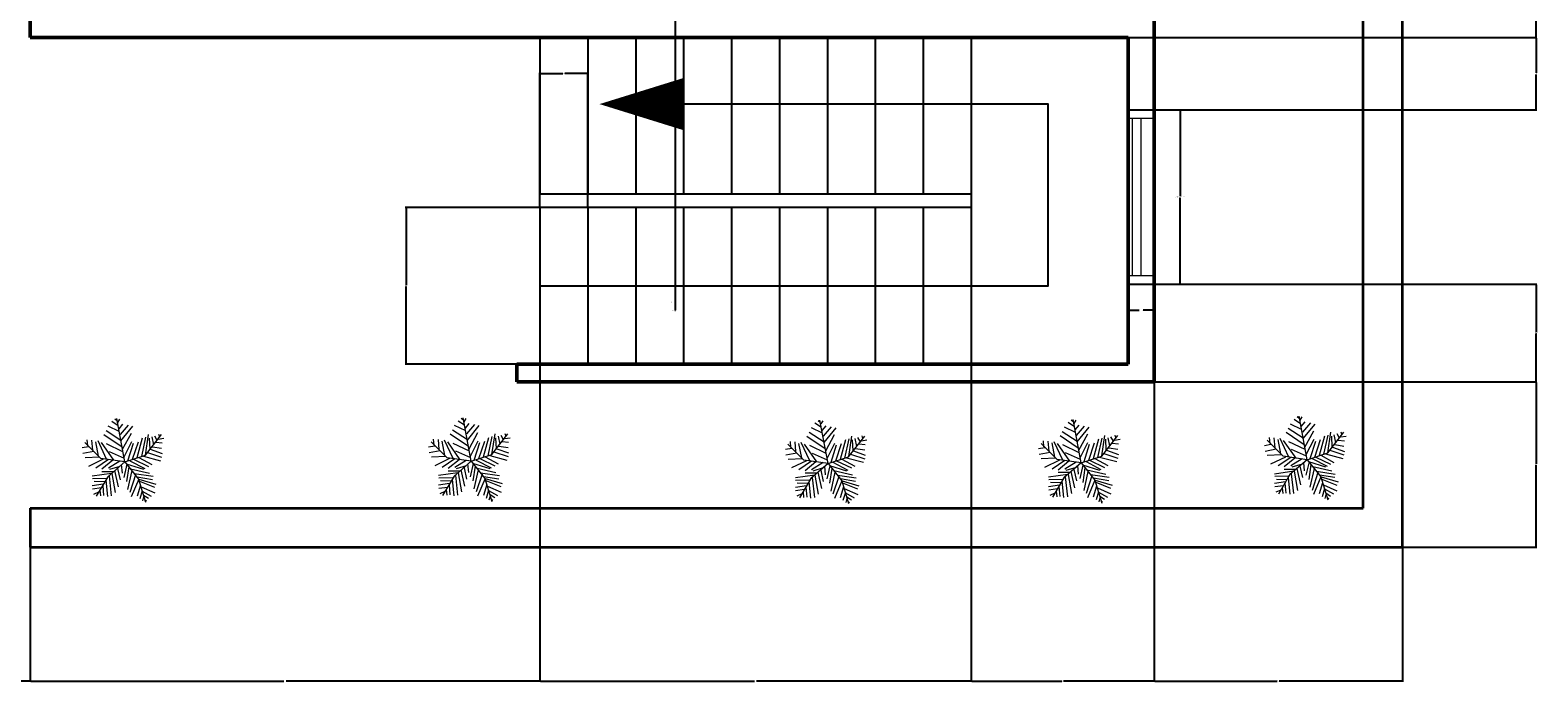
# Model space of a CAD drawing. Units: inches. Extents: x 156 to 720, y 11 to 679.
# Tile 2 of 5: x 374 to 720, y 11 to 161. Entities that reach past the tile are written whole.
import ezdxf

# ---------------------------------------------------------------- set-up
doc = ezdxf.new("R2010")
doc.units = ezdxf.units.IN
for name, color, linetype, lineweight in [('A-ANNO-DIMS', 2, 'Continuous', 18), ('A-FLOR-STRS', 7, 'Continuous', 25), ('A-GLAZ', 4, 'Continuous', 18), ('A-WALL', 7, 'Continuous', 50), ('C-PROP', 7, 'Continuous', 35), ('L-PLNT', 94, 'Continuous', 13)]:
    doc.layers.add(name, color=color, linetype=linetype, lineweight=lineweight)
doc.styles.get("Standard").update_dxf_attribs({"font": 'arial.ttf'})
doc.dimstyles.get("Standard").update_dxf_attribs({"dimtxt": 0.18, "dimasz": 0.18, "dimexe": 0.18, "dimexo": 0.0625, "dimgap": 0.09, "dimtad": 0, "dimtih": 1, "dimtoh": 1, "dimdec": 4, "dimzin": 0, "dimdsep": 46, "dimtxsty": 'Standard', "dimcen": 0.09, "dimadec": 0, "dimazin": 0, "dimtfac": 1, "dimtdec": 4, "dimtofl": 0, "dimtmove": 0, "dimatfit": 3, "dimfxl": 1, "dimtolj": 1, "dimtzin": 0, "dimarcsym": 0})

# ---------------------------------------------------------------- blocks, each defined once
blk = doc.blocks.new('*U13')
for p, q in [((-5.114, 28.097), (-24.676, 40.636)), ((-7.288, 39.707), (-21.778, 46.673)), ((-8.737, 47.138), (-17.069, 52.711)), ((-10.186, 53.64), (-13.084, 55.962)), ((0, 0), (-10.5, 57)), ((-9.099, 51.782), (-6.563, 55.962)), ((-7.65, 43.423), (-2.578, 49.46)), ((-5.839, 35.992), (4.667, 48.067)), ((-5.114, 27.632), (10.463, 46.673)), ((-31.5, 4.5), (-52.5, 25.5)), ((-48.585, 21.131), (-49.309, 29.026)), ((-43.513, 28.561), (-42.427, 15.558)), ((-38.442, 26.239), (-34.819, 7.663)), ((-35.544, 28.097), (-24.314, 3.947)), ((-14.533, 2.09), (-30.834, 25.31)), ((-3.665, 19.273), (-27.574, 35.527)), ((-24.314, 23.917), (-2.941, 13.7)), ((-2.941, 16.486), (8.652, 37.85)), ((-1.129, 6.734), (9.014, 26.704)), ((3.942, 1.625), (11.187, 24.381)), ((10.101, 3.483), (17.708, 26.239)), ((16.259, 5.805), (23.142, 31.348)), ((22.055, 7.198), (27.489, 32.277)), ((27, 9), (48, 36)), ((27.127, 9.056), (31.112, 35.992)), ((31.836, 30.883), (32.561, 16.486)), ((35.096, 32.741), (37.27, 22.524)), ((38.719, 34.134), (41.979, 28.561)), ((40.53, 25.775), (48.862, 24.846)), ((43.791, 29.954), (51.036, 30.883)), ((44.153, 36.456), (45.239, 32.741)), ((-47.498, 19.737), (-55.83, 18.344)), ((-40.615, 13.7), (-55.105, 10.913)), ((-33.37, 6.269), (-52.207, 5.34)), ((-28.299, 3.483), (-47.86, -5.805)), ((-21.416, 3.018), (-38.079, -8.128)), ((0, 0), (-31.5, 4.5)), ((-15.982, 2.09), (-30.11, -9.521)), ((0, 0), (-22.5, -19.5)), ((-6.563, 1.161), (-21.416, -8.128)), ((-20.691, 13.7), (-1.129, 4.876)), ((0, 0), (27, 9)), ((0, 0), (18, -22.5)), ((6.478, 1.625), (26.04, -8.592)), ((11.187, 3.483), (30.749, -5.805)), ((18.07, 5.805), (35.096, -3.483)), ((24.229, 7.663), (46.688, 1.625)), ((29.662, 12.307), (48.137, 6.269)), ((33.285, 16.486), (48.862, 10.913)), ((36.183, 19.737), (48.137, 17.88)), ((-17.431, -15.094), (-42.789, -18.809)), ((-22.5, -19.5), (-37.5, -45)), ((-15.257, -12.772), (-30.11, -12.772)), ((-20.691, -18.345), (-17.793, -44.352)), ((-6.563, -5.805), (-19.967, -9.985)), ((-17.069, -15.094), (-12.721, -40.172)), ((-13.446, -11.378), (-8.737, -32.741)), ((-9.461, -8.592), (-6.201, -23.453)), ((-4.752, -3.483), (-3.665, -14.629)), ((2.493, -3.019), (-1.491, -20.202)), ((1.769, -2.555), (24.229, -9.521)), ((5.029, -6.27), (2.131, -25.775)), ((9.014, -11.378), (3.58, -35.992)), ((14.085, -16.951), (6.478, -40.172)), ((7.565, -9.056), (32.198, -14.629)), ((12.274, -15.094), (36.907, -18.809)), ((16.259, -19.738), (36.183, -22.989)), ((-28.299, -29.026), (-42.789, -31.348)), ((-24.314, -21.596), (-42.427, -22.06)), ((-30.834, -34.135), (-42.427, -35.528)), ((-26.849, -26.24), (-40.253, -25.775)), ((-32.646, -36.921), (-31.921, -44.352)), ((-29.023, -30.884), (-27.936, -43.887)), ((-25.038, -23.918), (-22.865, -45.281)), ((18.07, -22.524), (8.289, -45.745)), ((20.244, -30.419), (15.897, -44.816)), ((18, -22.5), (27, -52.5)), ((18.433, -22.524), (40.53, -29.026)), ((19.157, -25.311), (38.719, -33.206)), ((22.78, -37.85), (19.519, -48.532)), ((21.331, -32.741), (39.081, -40.636)), ((22.78, -38.314), (34.372, -44.816)), ((-34.457, -39.708), (-40.978, -42.494)), ((24.591, -45.745), (23.142, -50.854)), ((24.591, -43.423), (30.749, -47.603)), ((26.764, -49.925), (28.213, -50.854))]:
    blk.add_line(p, q)
blk = doc.blocks.new('WIN-36IN-WALL6')
for p, q in [((6, 40), (0, 40)), ((6, 38), (0, 38)), ((0, 38), (0, 2)), ((1, 2), (1, 38)), ((3, 2), (3, 38)), ((6, 2), (6, 38)), ((0, 2), (6, 2)), ((0, 0), (6, 0))]:
    blk.add_line(p, q)
blk = doc.blocks.new('*D33')
at = {"layer": 'A-ANNO-DIMS', "color": 0, "lineweight": -2, "transparency": 16777216}
for p, q in [((631.79, 142.54), (637.9, 142.54)), ((637.72, 142.36), (637.72, 122.73)), ((637.72, 102.72), (637.72, 122.36)), ((631.79, 102.54), (637.9, 102.54))]:
    blk.add_line(p, q, dxfattribs=at)
at = {"layer": 'A-ANNO-DIMS', "color": 0, "transparency": 16777216}
for points in [[(637.69, 142.36), (637.75, 142.36), (637.72, 142.54)], [(637.69, 102.72), (637.75, 102.72), (637.72, 102.54)]]:
    blk.add_solid(points, dxfattribs=at)
at = {"layer": 'Defpoints', "color": 0, "transparency": 16777216}
for p in [(631.72, 142.54), (637.72, 142.54), (631.72, 102.54)]:
    blk.add_point(p, dxfattribs=at)
at = {"layer": 'A-ANNO-DIMS', "color": 0, "transparency": 16777216, "insert": (637.72, 122.54), "char_height": 0.18, "attachment_point": 5}
blk.add_mtext('\\A1;WINDOW C 40 TYP.', dxfattribs=at)
blk = doc.blocks.new('*D34')
at = {"layer": 'A-ANNO-DIMS', "color": 0, "lineweight": -2, "transparency": 16777216}
for p, q in [((625.72, 102.48), (625.72, 96.36)), ((631.72, 102.48), (631.72, 96.36)), ((625.9, 96.54), (628.26, 96.54)), ((631.54, 96.54), (629.18, 96.54))]:
    blk.add_line(p, q, dxfattribs=at)
at = {"layer": 'A-ANNO-DIMS', "color": 0, "transparency": 16777216}
for points in [[(625.9, 96.57), (625.9, 96.51), (625.72, 96.54)], [(631.54, 96.57), (631.54, 96.51), (631.72, 96.54)]]:
    blk.add_solid(points, dxfattribs=at)
at = {"layer": 'Defpoints', "color": 0, "transparency": 16777216}
for p in [(625.72, 102.54), (631.72, 102.54), (631.72, 96.54)]:
    blk.add_point(p, dxfattribs=at)
at = {"layer": 'A-ANNO-DIMS', "color": 0, "transparency": 16777216, "insert": (628.72, 96.54), "char_height": 0.18, "attachment_point": 5}
blk.add_mtext('\\A1;6 TYP.', dxfattribs=at)
blk = doc.blocks.new('*D52')
at = {"layer": 'A-ANNO-DIMS', "color": 0, "lineweight": -2, "transparency": 16777216}
for p, q in [((241.72, 42.09), (241.72, 11.27)), ((373.72, 42.09), (373.72, 11.27)), ((241.9, 11.45), (307.44, 11.45)), ((373.54, 11.45), (308, 11.45))]:
    blk.add_line(p, q, dxfattribs=at)
at = {"layer": 'A-ANNO-DIMS', "color": 0, "transparency": 16777216}
for points in [[(241.9, 11.48), (241.9, 11.42), (241.72, 11.45)], [(373.54, 11.48), (373.54, 11.42), (373.72, 11.45)]]:
    blk.add_solid(points, dxfattribs=at)
at = {"layer": 'Defpoints', "color": 0, "transparency": 16777216}
for p in [(241.72, 42.15), (373.72, 42.15), (373.72, 11.45)]:
    blk.add_point(p, dxfattribs=at)
at = {"layer": 'A-ANNO-DIMS', "color": 0, "transparency": 16777216, "insert": (307.72, 11.45), "char_height": 0.18, "attachment_point": 5}
blk.add_mtext('\\A1;132', dxfattribs=at)
blk = doc.blocks.new('*D53')
at = {"layer": 'A-ANNO-DIMS', "color": 0, "lineweight": -2, "transparency": 16777216}
for p, q in [((490.72, 84.09), (490.72, 11.27)), ((373.72, 42.09), (373.72, 11.27)), ((373.9, 11.45), (431.94, 11.45)), ((490.54, 11.45), (432.5, 11.45))]:
    blk.add_line(p, q, dxfattribs=at)
at = {"layer": 'A-ANNO-DIMS', "color": 0, "transparency": 16777216}
for points in [[(373.9, 11.48), (373.9, 11.42), (373.72, 11.45)], [(490.54, 11.48), (490.54, 11.42), (490.72, 11.45)]]:
    blk.add_solid(points, dxfattribs=at)
at = {"layer": 'Defpoints', "color": 0, "transparency": 16777216}
for p in [(490.72, 84.15), (373.72, 42.15), (490.72, 11.45)]:
    blk.add_point(p, dxfattribs=at)
at = {"layer": 'A-ANNO-DIMS', "color": 0, "transparency": 16777216, "insert": (432.22, 11.45), "char_height": 0.18, "attachment_point": 5}
blk.add_mtext('\\A1;117', dxfattribs=at)
blk = doc.blocks.new('*D54')
at = {"layer": 'A-ANNO-DIMS', "color": 0, "lineweight": -2, "transparency": 16777216}
for p, q in [((490.72, 84.09), (490.72, 11.27)), ((589.72, 84.09), (589.72, 11.27)), ((490.9, 11.45), (540, 11.45)), ((589.54, 11.45), (540.44, 11.45))]:
    blk.add_line(p, q, dxfattribs=at)
at = {"layer": 'A-ANNO-DIMS', "color": 0, "transparency": 16777216}
for points in [[(490.9, 11.48), (490.9, 11.42), (490.72, 11.45)], [(589.54, 11.48), (589.54, 11.42), (589.72, 11.45)]]:
    blk.add_solid(points, dxfattribs=at)
at = {"layer": 'Defpoints', "color": 0, "transparency": 16777216}
for p in [(490.72, 84.15), (589.72, 84.15), (589.72, 11.45)]:
    blk.add_point(p, dxfattribs=at)
at = {"layer": 'A-ANNO-DIMS', "color": 0, "transparency": 16777216, "insert": (540.22, 11.45), "char_height": 0.18, "attachment_point": 5}
blk.add_mtext('\\A1;99', dxfattribs=at)
blk = doc.blocks.new('*D55')
at = {"layer": 'A-ANNO-DIMS', "color": 0, "lineweight": -2, "transparency": 16777216}
for p, q in [((589.72, 84.09), (589.72, 11.27)), ((631.72, 80.09), (631.72, 11.27)), ((589.9, 11.45), (610.5, 11.45)), ((631.54, 11.45), (610.95, 11.45))]:
    blk.add_line(p, q, dxfattribs=at)
at = {"layer": 'A-ANNO-DIMS', "color": 0, "transparency": 16777216}
for points in [[(589.9, 11.48), (589.9, 11.42), (589.72, 11.45)], [(631.54, 11.48), (631.54, 11.42), (631.72, 11.45)]]:
    blk.add_solid(points, dxfattribs=at)
at = {"layer": 'Defpoints', "color": 0, "transparency": 16777216}
for p in [(589.72, 84.15), (631.72, 80.15), (631.72, 11.45)]:
    blk.add_point(p, dxfattribs=at)
at = {"layer": 'A-ANNO-DIMS', "color": 0, "transparency": 16777216, "insert": (610.72, 11.45), "char_height": 0.18, "attachment_point": 5}
blk.add_mtext('\\A1;42', dxfattribs=at)
blk = doc.blocks.new('*D56')
at = {"layer": 'A-ANNO-DIMS', "color": 0, "lineweight": -2, "transparency": 16777216}
for p, q in [((631.72, 80.09), (631.72, 11.27)), ((688.72, 42.09), (688.72, 11.27)), ((631.9, 11.45), (660, 11.45)), ((688.54, 11.45), (660.44, 11.45))]:
    blk.add_line(p, q, dxfattribs=at)
at = {"layer": 'A-ANNO-DIMS', "color": 0, "transparency": 16777216}
for points in [[(631.9, 11.48), (631.9, 11.42), (631.72, 11.45)], [(688.54, 11.48), (688.54, 11.42), (688.72, 11.45)]]:
    blk.add_solid(points, dxfattribs=at)
at = {"layer": 'Defpoints', "color": 0, "transparency": 16777216}
for p in [(631.72, 80.15), (688.72, 42.15), (688.72, 11.45)]:
    blk.add_point(p, dxfattribs=at)
at = {"layer": 'A-ANNO-DIMS', "color": 0, "transparency": 16777216, "insert": (660.22, 11.45), "char_height": 0.18, "attachment_point": 5}
blk.add_mtext('\\A1;57', dxfattribs=at)
blk = doc.blocks.new('*D57')
at = {"layer": 'A-ANNO-DIMS', "color": 0, "lineweight": -2, "transparency": 16777216}
for p, q in [((631.79, 80.15), (719.6, 80.15)), ((719.42, 79.97), (719.42, 61.33)), ((719.42, 42.33), (719.42, 60.97)), ((688.79, 42.15), (719.6, 42.15))]:
    blk.add_line(p, q, dxfattribs=at)
at = {"layer": 'A-ANNO-DIMS', "color": 0, "transparency": 16777216}
for points in [[(719.39, 79.97), (719.45, 79.97), (719.42, 80.15)], [(719.39, 42.33), (719.45, 42.33), (719.42, 42.15)]]:
    blk.add_solid(points, dxfattribs=at)
at = {"layer": 'Defpoints', "color": 0, "transparency": 16777216}
for p in [(631.72, 80.15), (719.42, 80.15), (688.72, 42.15)]:
    blk.add_point(p, dxfattribs=at)
at = {"layer": 'A-ANNO-DIMS', "color": 0, "transparency": 16777216, "insert": (719.42, 61.15), "char_height": 0.18, "attachment_point": 5}
blk.add_mtext('\\A1;38', dxfattribs=at)
blk = doc.blocks.new('*D58')
at = {"layer": 'A-ANNO-DIMS', "color": 0, "lineweight": -2, "transparency": 16777216}
for p, q in [((625.79, 102.54), (719.6, 102.54)), ((719.42, 102.36), (719.42, 91.53)), ((719.42, 80.33), (719.42, 91.17)), ((631.79, 80.15), (719.6, 80.15))]:
    blk.add_line(p, q, dxfattribs=at)
at = {"layer": 'A-ANNO-DIMS', "color": 0, "transparency": 16777216}
for points in [[(719.39, 102.36), (719.45, 102.36), (719.42, 102.54)], [(719.39, 80.33), (719.45, 80.33), (719.42, 80.15)]]:
    blk.add_solid(points, dxfattribs=at)
at = {"layer": 'Defpoints', "color": 0, "transparency": 16777216}
for p in [(625.72, 102.54), (719.42, 102.54), (631.72, 80.15)]:
    blk.add_point(p, dxfattribs=at)
at = {"layer": 'A-ANNO-DIMS', "color": 0, "transparency": 16777216, "insert": (719.42, 91.35), "char_height": 0.18, "attachment_point": 5}
blk.add_mtext('\\A1;22.39', dxfattribs=at)
blk = doc.blocks.new('*D59')
at = {"layer": 'A-ANNO-DIMS', "color": 0, "lineweight": -2, "transparency": 16777216}
for p, q in [((625.79, 159.15), (719.6, 159.15)), ((719.42, 158.97), (719.42, 151.03)), ((719.42, 142.72), (719.42, 150.67)), ((625.79, 142.54), (719.6, 142.54))]:
    blk.add_line(p, q, dxfattribs=at)
at = {"layer": 'A-ANNO-DIMS', "color": 0, "transparency": 16777216}
for points in [[(719.39, 158.97), (719.45, 158.97), (719.42, 159.15)], [(719.39, 142.72), (719.45, 142.72), (719.42, 142.54)]]:
    blk.add_solid(points, dxfattribs=at)
at = {"layer": 'Defpoints', "color": 0, "transparency": 16777216}
for p in [(625.72, 159.15), (719.42, 159.15), (625.72, 142.54)]:
    blk.add_point(p, dxfattribs=at)
at = {"layer": 'A-ANNO-DIMS', "color": 0, "transparency": 16777216, "insert": (719.42, 150.85), "char_height": 0.18, "attachment_point": 5}
blk.add_mtext('\\A1;16.608', dxfattribs=at)
blk = doc.blocks.new('*D60')
at = {"layer": 'A-ANNO-DIMS', "color": 0, "lineweight": -2, "transparency": 16777216}
for p, q in [((625.79, 215.4), (719.6, 215.4)), ((719.42, 215.22), (719.42, 187.46)), ((719.42, 159.33), (719.42, 187.09)), ((625.79, 159.15), (719.6, 159.15))]:
    blk.add_line(p, q, dxfattribs=at)
at = {"layer": 'A-ANNO-DIMS', "color": 0, "transparency": 16777216}
for points in [[(719.39, 215.22), (719.45, 215.22), (719.42, 215.4)], [(719.39, 159.33), (719.45, 159.33), (719.42, 159.15)]]:
    blk.add_solid(points, dxfattribs=at)
at = {"layer": 'Defpoints', "color": 0, "transparency": 16777216}
for p in [(625.72, 215.4), (719.42, 215.4), (625.72, 159.15)]:
    blk.add_point(p, dxfattribs=at)
at = {"layer": 'A-ANNO-DIMS', "color": 0, "transparency": 16777216, "insert": (719.42, 187.27), "char_height": 0.18, "attachment_point": 5}
blk.add_mtext('\\A1;56.25', dxfattribs=at)
blk = doc.blocks.new('*D77')
at = {"layer": 'A-ANNO-DIMS', "color": 0, "lineweight": -2, "transparency": 16777216}
for p, q in [((490.72, 120.21), (490.72, 151.03)), ((490.9, 150.85), (496.03, 150.85)), ((501.54, 150.85), (496.42, 150.85)), ((501.72, 120.21), (501.72, 151.03))]:
    blk.add_line(p, q, dxfattribs=at)
at = {"layer": 'A-ANNO-DIMS', "color": 0, "transparency": 16777216}
for points in [[(490.9, 150.88), (490.9, 150.82), (490.72, 150.85)], [(501.54, 150.88), (501.54, 150.82), (501.72, 150.85)]]:
    blk.add_solid(points, dxfattribs=at)
at = {"layer": 'Defpoints', "color": 0, "transparency": 16777216}
for p in [(501.72, 150.85), (490.72, 120.15), (501.72, 120.15)]:
    blk.add_point(p, dxfattribs=at)
at = {"layer": 'A-ANNO-DIMS', "color": 0, "transparency": 16777216, "insert": (496.22, 150.85), "char_height": 0.18, "attachment_point": 5}
blk.add_mtext('\\A1;11', dxfattribs=at)
blk = doc.blocks.new('*D78')
at = {"layer": 'A-ANNO-DIMS', "color": 0, "lineweight": -2, "transparency": 16777216}
for p, q in [((490.66, 120.15), (459.84, 120.15)), ((460.02, 119.97), (460.02, 102.33)), ((460.02, 84.33), (460.02, 101.97)), ((490.66, 84.15), (459.84, 84.15))]:
    blk.add_line(p, q, dxfattribs=at)
at = {"layer": 'A-ANNO-DIMS', "color": 0, "transparency": 16777216}
for points in [[(459.99, 119.97), (460.05, 119.97), (460.02, 120.15)], [(459.99, 84.33), (460.05, 84.33), (460.02, 84.15)]]:
    blk.add_solid(points, dxfattribs=at)
at = {"layer": 'Defpoints', "color": 0, "transparency": 16777216}
for p in [(460.02, 120.15), (490.72, 120.15), (490.72, 84.15)]:
    blk.add_point(p, dxfattribs=at)
at = {"layer": 'A-ANNO-DIMS', "color": 0, "transparency": 16777216, "insert": (460.02, 102.15), "char_height": 0.18, "attachment_point": 5}
blk.add_mtext('\\A1;36', dxfattribs=at)
blk = doc.blocks.new('*D81')
at = {"layer": 'A-ANNO-DIMS', "color": 0, "lineweight": -2, "transparency": 16777216}
for p, q in [((521.79, 292.35), (521.97, 292.35)), ((521.88, 292.26), (521.88, 292.44)), ((521.88, 98.43), (521.88, 170.97)), ((521.7, 98.43), (521.88, 98.43))]:
    blk.add_line(p, q, dxfattribs=at)
at = {"layer": 'A-ANNO-DIMS', "color": 0, "transparency": 16777216}
blk.add_solid([(521.85, 170.97), (521.91, 170.97), (521.88, 171.15)], dxfattribs=at)
at = {"layer": 'Defpoints', "color": 0, "transparency": 16777216}
for p in [(521.88, 292.35), (521.88, 171.15)]:
    blk.add_point(p, dxfattribs=at)
at = {"layer": 'A-ANNO-DIMS', "color": 0, "transparency": 16777216, "insert": (521.22, 98.43), "char_height": 0.18, "attachment_point": 5}
blk.add_mtext('\\A1;R121.2', dxfattribs=at)
blk = doc.blocks.new('*D82')
at = {"layer": 'A-ANNO-DIMS', "color": 0, "lineweight": -2, "transparency": 16777216}
for p, q in [((521.79, 279.4), (521.97, 279.4)), ((521.88, 279.31), (521.88, 279.49)), ((521.88, 96.6), (521.88, 164.97)), ((521.7, 96.6), (521.88, 96.6))]:
    blk.add_line(p, q, dxfattribs=at)
at = {"layer": 'A-ANNO-DIMS', "color": 0, "transparency": 16777216}
blk.add_solid([(521.85, 164.97), (521.91, 164.97), (521.88, 165.15)], dxfattribs=at)
at = {"layer": 'Defpoints', "color": 0, "transparency": 16777216}
for p in [(521.88, 279.4), (521.88, 165.15)]:
    blk.add_point(p, dxfattribs=at)
at = {"layer": 'A-ANNO-DIMS', "color": 0, "transparency": 16777216, "insert": (521.15, 96.6), "char_height": 0.18, "attachment_point": 5}
blk.add_mtext('\\A1;R114.25', dxfattribs=at)

msp = doc.modelspace()

# ---------------------------------------------------------------- linework, layer by layer
at = {"layer": 'A-FLOR-STRS'}
for p, q in [((490.7236, 159.1514), (490.7236, 123.1514)), ((501.7236, 159.1514), (501.7236, 123.1514)), ((512.7236, 159.1514), (512.7236, 123.1514)), ((523.7236, 159.1514), (523.7236, 123.1514)), ((534.7236, 159.1514), (534.7236, 123.1514)), ((545.7236, 159.1514), (545.7236, 123.1514)), ((556.7236, 159.1514), (556.7236, 123.1514)), ((567.7236, 159.1514), (567.7236, 123.1514)), ((578.7236, 159.1514), (578.7236, 123.1514)), ((589.7236, 159.1514), (589.7236, 84.1514)), ((589.7236, 123.1514), (490.7236, 123.1514)), ((589.7236, 120.1514), (490.7236, 120.1514)), ((490.7236, 120.1514), (490.7236, 84.1514)), ((501.7236, 120.1514), (501.7236, 84.1514)), ((512.7236, 120.1514), (512.7236, 84.1514)), ((523.7236, 120.1514), (523.7236, 84.1514)), ((534.7236, 120.1514), (534.7236, 84.1514)), ((545.7236, 120.1514), (545.7236, 84.1514)), ((556.7236, 120.1514), (556.7236, 84.1514)), ((567.7236, 120.1514), (567.7236, 84.1514)), ((578.7236, 120.1514), (578.7236, 84.1514))]:
    msp.add_line(p, q, dxfattribs=at)
msp.add_lwpolyline([(523.7236, 143.8512, 12, 0, 0), (504.4149, 143.8512, 0, 0, 0)], format="xyseb", dxfattribs=at)
msp.add_lwpolyline([(490.7236, 102.1514), (607.4278, 102.1514), (607.4278, 143.8512), (523.7236, 143.8512)], dxfattribs=at)
at = {"layer": 'A-WALL'}
for p, q in [((631.7236, 453.1514), (631.7236, 80.1514)), ((373.7236, 204.1514), (373.7236, 159.1514)), ((625.7236, 159.1514), (373.7236, 159.1514)), ((625.7236, 159.1514), (625.7236, 84.1514)), ((625.7236, 84.1514), (485.3985, 84.1514)), ((485.3985, 84.1514), (485.3985, 80.1514)), ((631.7236, 80.1514), (485.3985, 80.1514))]:
    msp.add_line(p, q, dxfattribs=at)
at = {"layer": 'C-PROP'}
for p, q in [((688.7236, 42.1514), (688.7236, 642.1514)), ((679.7236, 51.1514), (679.7236, 543.1514)), ((373.7236, 51.1514), (679.7236, 51.1514)), ((373.7236, 51.1514), (373.7236, 42.1514)), ((373.7236, 42.1514), (688.7236, 42.1514))]:
    msp.add_line(p, q, dxfattribs=at)

# ---------------------------------------------------------------- block references
at = {"layer": 'A-GLAZ'}
msp.add_blockref('WIN-36IN-WALL6', (625.724, 102.543), dxfattribs=at)
at = {"layer": 'L-PLNT', "xscale": 0.175286236255467, "yscale": 0.175286236255467, "zscale": 0.175286236255467}
for p in [(395.4685, 61.7379), (474.9726, 61.8845), (556.8636, 61.3643), (614.956, 61.512), (666.84, 62.2504)]:
    msp.add_blockref('*U13', p, dxfattribs=at)

# ---------------------------------------------------------------- dimensions: what is measured, and where the dimension line sits
at = {"layer": 'A-ANNO-DIMS'}
for center, mpoint, override, picture, middle in [((521.881, 292.3482), (521.881, 171.1514), {"dimdec": 1, "dimlfac": 1, "dimrnd": 0, "dimzin": 0, "dimdsep": 46, "dimlunit": 2}, '*D81', (521.2221, 98.4333)), ((521.881, 279.4014), (521.881, 165.1514), {"dimdec": 2, "dimlfac": 1, "dimrnd": 0, "dimzin": 0, "dimdsep": 46, "dimlunit": 2}, '*D82', (521.1506, 96.6014))]:
    dim = msp.add_radius_dim(center=center, mpoint=mpoint, dimstyle='Standard', override=override, dxfattribs=at)
    dim.commit()
    dim.dimension.update_dxf_attribs({"geometry": picture, "text_midpoint": middle, "dimtype": 164})
for base, p1, p2, override, picture, middle in [((719.4236, 215.3977), (625.7236, 159.1514), (625.7236, 215.3977), {"dimdec": 2, "dimlfac": 1, "dimrnd": 0, "dimzin": 0, "dimdsep": 46, "dimlunit": 2}, '*D60', (719.4236, 187.2746)), ((719.4236, 159.1514), (625.7236, 142.5434), (625.7236, 159.1514), {"dimdec": 3, "dimlfac": 1, "dimrnd": 0, "dimzin": 0, "dimdsep": 46, "dimlunit": 2}, '*D59', (719.4236, 150.8474)), ((460.0236, 120.1514), (490.7236, 84.1514), (490.7236, 120.1514), {"dimdec": 0, "dimlfac": 1, "dimrnd": 0, "dimzin": 0, "dimdsep": 46, "dimlunit": 2}, '*D78', (460.0236, 102.1514)), ((719.4236, 102.5434), (631.7236, 80.1514), (625.7236, 102.5434), {"dimdec": 2, "dimlfac": 1, "dimrnd": 0, "dimzin": 0, "dimdsep": 46, "dimlunit": 2}, '*D58', (719.4236, 91.3474)), ((719.4236, 80.1514), (688.7236, 42.1514), (631.7236, 80.1514), {"dimdec": 0, "dimlfac": 1, "dimrnd": 0, "dimzin": 0, "dimdsep": 46, "dimlunit": 2}, '*D57', (719.4236, 61.1514))]:
    dim = msp.add_linear_dim(base=base, p1=p1, p2=p2, angle=90, dimstyle='Standard', override=override, dxfattribs=at)
    dim.commit()
    dim.dimension.update_dxf_attribs({"geometry": picture, "text_midpoint": middle})
for base, p1, p2, picture, middle in [((501.7236, 150.8514), (490.7236, 120.1514), (501.7236, 120.1514), '*D77', (496.2236, 150.8514)), ((490.7236, 11.4514), (373.7236, 42.1514), (490.7236, 84.1514), '*D53', (432.2236, 11.4514)), ((589.7236, 11.4514), (490.7236, 84.1514), (589.7236, 84.1514), '*D54', (540.2236, 11.4514)), ((631.7236, 11.4514), (589.7236, 84.1514), (631.7236, 80.1514), '*D55', (610.7236, 11.4514)), ((688.7236, 11.4514), (631.7236, 80.1514), (688.7236, 42.1514), '*D56', (660.2236, 11.4514)), ((373.7236, 11.4514), (241.7236, 42.1514), (373.7236, 42.1514), '*D52', (307.7236, 11.4514))]:
    dim = msp.add_linear_dim(base=base, p1=p1, p2=p2, dimstyle='Standard', override={"dimdec": 0, "dimlfac": 1, "dimrnd": 0, "dimzin": 0, "dimdsep": 46, "dimlunit": 2}, dxfattribs=at)
    dim.commit()
    dim.dimension.update_dxf_attribs({"geometry": picture, "text_midpoint": middle})
dim = msp.add_linear_dim(base=(637.7236, 142.5434), p1=(631.7236, 102.5434), p2=(631.7236, 142.5434), angle=90, text='WINDOW C <> TYP.', dimstyle='Standard', override={"dimdec": 0, "dimlfac": 1, "dimrnd": 0, "dimzin": 0, "dimdsep": 46, "dimlunit": 2}, dxfattribs=at)
dim.commit()
dim.dimension.update_dxf_attribs({"geometry": '*D33', "text_midpoint": (637.7236, 122.5434)})
dim = msp.add_linear_dim(base=(631.7236, 96.5434), p1=(625.7236, 102.5434), p2=(631.7236, 102.5434), text='<> TYP.', dimstyle='Standard', override={"dimdec": 0, "dimlfac": 1, "dimrnd": 0, "dimzin": 0, "dimdsep": 46, "dimlunit": 2}, dxfattribs=at)
dim.commit()
dim.dimension.update_dxf_attribs({"geometry": '*D34', "text_midpoint": (628.7236, 96.5434)})

doc.saveas('drawing.dxf')
